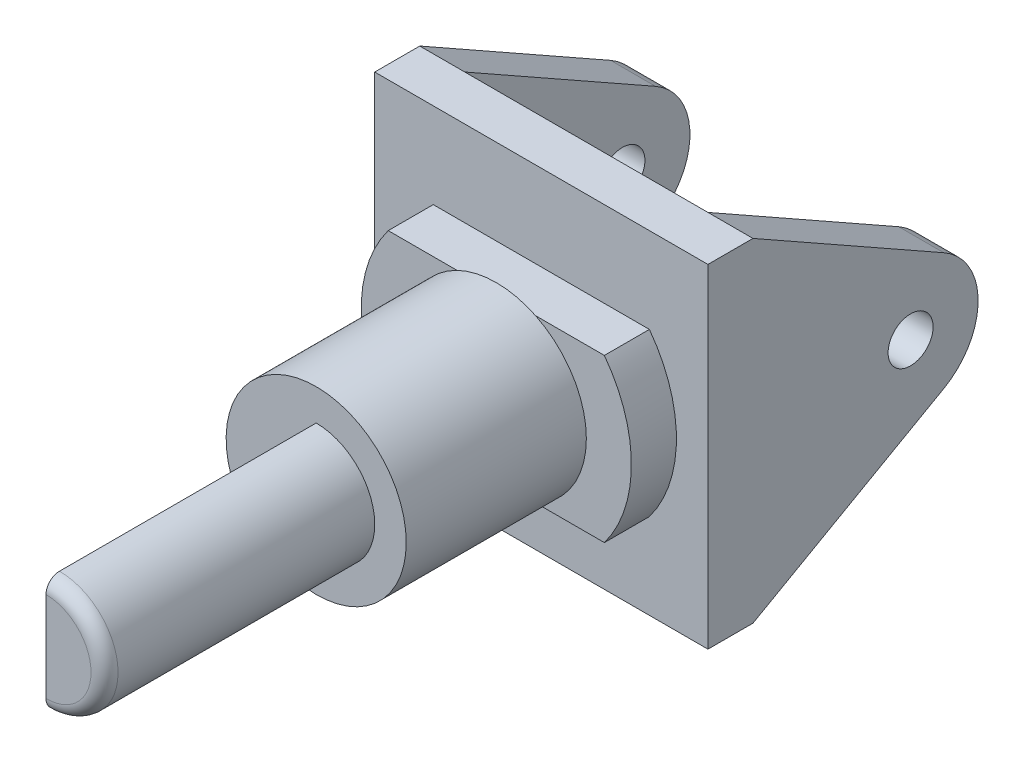
ISO-10303-21;
HEADER;
FILE_DESCRIPTION(('STEP AP214'),'2;1');
FILE_NAME('part.step','',(''),(''),'','','');
FILE_SCHEMA(('AUTOMOTIVE_DESIGN { 1 0 10303 214 1 1 1 1 }'));
ENDSEC;
DATA;
#1=APPLICATION_CONTEXT('core data for automotive mechanical design processes');
#2=APPLICATION_PROTOCOL_DEFINITION('international standard','automotive_design',2000,#1);
#3=PRODUCT_CONTEXT('',#1,'mechanical');
#4=PRODUCT('Part','Part','',(#3));
#5=PRODUCT_RELATED_PRODUCT_CATEGORY('part','',(#4));
#6=PRODUCT_DEFINITION_FORMATION('','',#4);
#7=PRODUCT_DEFINITION_CONTEXT('part definition',#1,'design');
#8=PRODUCT_DEFINITION('design','',#6,#7);
#9=PRODUCT_DEFINITION_SHAPE('','',#8);
#10=(LENGTH_UNIT() NAMED_UNIT(*) SI_UNIT(.MILLI.,.METRE.));
#11=(NAMED_UNIT(*) PLANE_ANGLE_UNIT() SI_UNIT($,.RADIAN.));
#12=(NAMED_UNIT(*) SI_UNIT($,.STERADIAN.) SOLID_ANGLE_UNIT());
#13=UNCERTAINTY_MEASURE_WITH_UNIT(LENGTH_MEASURE(1.E-05),#10,'distance_accuracy_value','');
#14=(GEOMETRIC_REPRESENTATION_CONTEXT(3) GLOBAL_UNCERTAINTY_ASSIGNED_CONTEXT((#13)) GLOBAL_UNIT_ASSIGNED_CONTEXT((#10,
#11,#12)) REPRESENTATION_CONTEXT('',''));
#15=CARTESIAN_POINT('',(0.,0.,0.));
#16=DIRECTION('',(0.,0.,1.));
#17=DIRECTION('',(1.,0.,0.));
#18=AXIS2_PLACEMENT_3D('',#15,#16,#17);
#19=CARTESIAN_POINT('',(0.,0.,-10.));
#20=DIRECTION('',(0.,0.,-1.));
#21=DIRECTION('',(-1.,0.,0.));
#22=AXIS2_PLACEMENT_3D('',#19,#20,#21);
#23=PLANE('',#22);
#24=DIRECTION('',(-1.,0.,0.));
#25=VECTOR('',#24,1.);
#26=CARTESIAN_POINT('',(37.,-37.,-10.));
#27=LINE('',#26,#25);
#28=CARTESIAN_POINT('',(27.,-37.,-10.));
#29=VERTEX_POINT('',#28);
#30=CARTESIAN_POINT('',(-27.,-37.,-10.));
#31=VERTEX_POINT('',#30);
#32=EDGE_CURVE('E238',#29,#31,#27,.T.);
#33=ORIENTED_EDGE('',*,*,#32,.T.);
#34=DIRECTION('',(0.,-1.,0.));
#35=VECTOR('',#34,1.);
#36=CARTESIAN_POINT('',(-27.,37.,-10.));
#37=LINE('',#36,#35);
#38=CARTESIAN_POINT('',(-27.,37.,-10.));
#39=VERTEX_POINT('',#38);
#40=EDGE_CURVE('E54',#39,#31,#37,.T.);
#41=ORIENTED_EDGE('',*,*,#40,.F.);
#42=DIRECTION('',(1.,0.,0.));
#43=VECTOR('',#42,1.);
#44=CARTESIAN_POINT('',(37.,37.,-10.));
#45=LINE('',#44,#43);
#46=CARTESIAN_POINT('',(27.,37.,-10.));
#47=VERTEX_POINT('',#46);
#48=EDGE_CURVE('E237',#39,#47,#45,.T.);
#49=ORIENTED_EDGE('',*,*,#48,.T.);
#50=DIRECTION('',(0.,-1.,0.));
#51=VECTOR('',#50,1.);
#52=CARTESIAN_POINT('',(27.,37.,-10.));
#53=LINE('',#52,#51);
#54=EDGE_CURVE('E208',#47,#29,#53,.T.);
#55=ORIENTED_EDGE('',*,*,#54,.T.);
#56=EDGE_LOOP('',(#33,#41,#49,#55));
#57=FACE_BOUND('',#56,.T.);
#58=ADVANCED_FACE('F39',(#57),#23,.T.);
#59=CARTESIAN_POINT('',(0.,0.,110.));
#60=DIRECTION('',(0.,0.,-1.));
#61=DIRECTION('',(-1.,0.,0.));
#62=AXIS2_PLACEMENT_3D('',#59,#60,#61);
#63=CYLINDRICAL_SURFACE('',#62,13.);
#64=DIRECTION('',(0.,0.,-1.));
#65=VECTOR('',#64,1.);
#66=CARTESIAN_POINT('',(0.,13.,110.));
#67=LINE('',#66,#65);
#68=CARTESIAN_POINT('',(0.,13.,107.));
#69=VERTEX_POINT('',#68);
#70=CARTESIAN_POINT('',(0.,13.,50.));
#71=VERTEX_POINT('',#70);
#72=EDGE_CURVE('E269',#69,#71,#67,.T.);
#73=ORIENTED_EDGE('',*,*,#72,.F.);
#74=CARTESIAN_POINT('',(0.,0.,107.));
#75=DIRECTION('',(0.,0.,1.));
#76=DIRECTION('',(1.,0.,0.));
#77=AXIS2_PLACEMENT_3D('',#74,#75,#76);
#78=CIRCLE('',#77,13.);
#79=CARTESIAN_POINT('',(0.,-13.,107.));
#80=VERTEX_POINT('',#79);
#81=EDGE_CURVE('E325',#69,#80,#78,.F.);
#82=ORIENTED_EDGE('',*,*,#81,.T.);
#83=DIRECTION('',(0.,0.,-1.));
#84=VECTOR('',#83,1.);
#85=CARTESIAN_POINT('',(0.,-13.,110.));
#86=LINE('',#85,#84);
#87=CARTESIAN_POINT('',(0.,-13.,50.));
#88=VERTEX_POINT('',#87);
#89=EDGE_CURVE('E272',#88,#80,#86,.F.);
#90=ORIENTED_EDGE('',*,*,#89,.F.);
#91=CARTESIAN_POINT('',(0.,0.,50.));
#92=DIRECTION('',(0.,0.,1.));
#93=DIRECTION('',(1.,0.,0.));
#94=AXIS2_PLACEMENT_3D('',#91,#92,#93);
#95=CIRCLE('',#94,13.);
#96=EDGE_CURVE('E274',#88,#71,#95,.T.);
#97=ORIENTED_EDGE('',*,*,#96,.T.);
#98=EDGE_LOOP('',(#73,#82,#90,#97));
#99=FACE_BOUND('',#98,.T.);
#100=ADVANCED_FACE('F337',(#99),#63,.T.);
#101=CARTESIAN_POINT('',(0.,0.,110.));
#102=DIRECTION('',(0.,0.,1.));
#103=DIRECTION('',(1.,0.,0.));
#104=AXIS2_PLACEMENT_3D('',#101,#102,#103);
#105=PLANE('',#104);
#106=CARTESIAN_POINT('',(0.,0.,110.));
#107=DIRECTION('',(0.,0.,1.));
#108=DIRECTION('',(1.,0.,0.));
#109=AXIS2_PLACEMENT_3D('',#106,#107,#108);
#110=CIRCLE('',#109,10.);
#111=CARTESIAN_POINT('',(0.,-10.,110.));
#112=VERTEX_POINT('',#111);
#113=CARTESIAN_POINT('',(0.,10.,110.));
#114=VERTEX_POINT('',#113);
#115=EDGE_CURVE('E280',#112,#114,#110,.T.);
#116=ORIENTED_EDGE('',*,*,#115,.T.);
#117=DIRECTION('',(0.,-1.,0.));
#118=VECTOR('',#117,1.);
#119=CARTESIAN_POINT('',(0.,0.,110.));
#120=LINE('',#119,#118);
#121=EDGE_CURVE('E268',#114,#112,#120,.T.);
#122=ORIENTED_EDGE('',*,*,#121,.T.);
#123=EDGE_LOOP('',(#116,#122));
#124=FACE_BOUND('',#123,.T.);
#125=ADVANCED_FACE('F335',(#124),#105,.T.);
#126=CARTESIAN_POINT('',(0.,0.,107.));
#127=DIRECTION('',(0.,0.,1.));
#128=DIRECTION('',(1.,0.,0.));
#129=AXIS2_PLACEMENT_3D('',#126,#127,#128);
#130=TOROIDAL_SURFACE('',#129,10.,3.);
#131=ORIENTED_EDGE('',*,*,#115,.F.);
#132=CARTESIAN_POINT('',(0.,-10.,107.));
#133=DIRECTION('',(-1.,0.,0.));
#134=DIRECTION('',(0.,0.,1.));
#135=AXIS2_PLACEMENT_3D('',#132,#133,#134);
#136=CIRCLE('',#135,3.);
#137=EDGE_CURVE('E11',#112,#80,#136,.F.);
#138=ORIENTED_EDGE('',*,*,#137,.T.);
#139=ORIENTED_EDGE('',*,*,#81,.F.);
#140=CARTESIAN_POINT('',(0.,10.,107.));
#141=DIRECTION('',(-1.,0.,0.));
#142=DIRECTION('',(0.,0.,1.));
#143=AXIS2_PLACEMENT_3D('',#140,#141,#142);
#144=CIRCLE('',#143,3.);
#145=EDGE_CURVE('E48',#69,#114,#144,.F.);
#146=ORIENTED_EDGE('',*,*,#145,.T.);
#147=EDGE_LOOP('',(#131,#138,#139,#146));
#148=FACE_BOUND('',#147,.T.);
#149=ADVANCED_FACE('F41',(#148),#130,.T.);
#150=CARTESIAN_POINT('',(0.,0.,10.));
#151=DIRECTION('',(0.,0.,1.));
#152=DIRECTION('',(1.,0.,0.));
#153=AXIS2_PLACEMENT_3D('',#150,#151,#152);
#154=PLANE('',#153);
#155=CARTESIAN_POINT('',(0.,0.,10.));
#156=DIRECTION('',(0.,0.,1.));
#157=DIRECTION('',(1.,0.,0.));
#158=AXIS2_PLACEMENT_3D('',#155,#156,#157);
#159=CIRCLE('',#158,20.);
#160=CARTESIAN_POINT('',(-8.71779788708135,18.,10.));
#161=VERTEX_POINT('',#160);
#162=CARTESIAN_POINT('',(-8.71779788708135,-18.,10.));
#163=VERTEX_POINT('',#162);
#164=EDGE_CURVE('E279',#161,#163,#159,.T.);
#165=ORIENTED_EDGE('',*,*,#164,.F.);
#166=DIRECTION('',(1.,0.,0.));
#167=VECTOR('',#166,1.);
#168=CARTESIAN_POINT('',(0.,18.,10.));
#169=LINE('',#168,#167);
#170=CARTESIAN_POINT('',(-24.,18.,10.));
#171=VERTEX_POINT('',#170);
#172=EDGE_CURVE('E293',#171,#161,#169,.T.);
#173=ORIENTED_EDGE('',*,*,#172,.F.);
#174=CARTESIAN_POINT('',(0.,0.,10.));
#175=DIRECTION('',(0.,0.,1.));
#176=DIRECTION('',(1.,0.,0.));
#177=AXIS2_PLACEMENT_3D('',#174,#175,#176);
#178=CIRCLE('',#177,30.);
#179=CARTESIAN_POINT('',(-24.,-18.,10.));
#180=VERTEX_POINT('',#179);
#181=EDGE_CURVE('E317',#171,#180,#178,.T.);
#182=ORIENTED_EDGE('',*,*,#181,.T.);
#183=DIRECTION('',(-1.,0.,0.));
#184=VECTOR('',#183,1.);
#185=CARTESIAN_POINT('',(0.,-18.,10.));
#186=LINE('',#185,#184);
#187=EDGE_CURVE('E282',#163,#180,#186,.T.);
#188=ORIENTED_EDGE('',*,*,#187,.F.);
#189=EDGE_LOOP('',(#165,#173,#182,#188));
#190=FACE_BOUND('',#189,.T.);
#191=ADVANCED_FACE('F377',(#190),#154,.T.);
#192=CARTESIAN_POINT('',(0.,0.,10.));
#193=DIRECTION('',(0.,0.,-1.));
#194=DIRECTION('',(-1.,0.,0.));
#195=AXIS2_PLACEMENT_3D('',#192,#193,#194);
#196=CYLINDRICAL_SURFACE('',#195,30.);
#197=ORIENTED_EDGE('',*,*,#181,.F.);
#198=DIRECTION('',(0.,0.,1.));
#199=VECTOR('',#198,1.);
#200=CARTESIAN_POINT('',(-24.,18.,0.));
#201=LINE('',#200,#199);
#202=CARTESIAN_POINT('',(-24.,18.,0.));
#203=VERTEX_POINT('',#202);
#204=EDGE_CURVE('E298',#203,#171,#201,.T.);
#205=ORIENTED_EDGE('',*,*,#204,.F.);
#206=CARTESIAN_POINT('',(0.,0.,0.));
#207=DIRECTION('',(0.,0.,1.));
#208=DIRECTION('',(1.,0.,0.));
#209=AXIS2_PLACEMENT_3D('',#206,#207,#208);
#210=CIRCLE('',#209,30.);
#211=CARTESIAN_POINT('',(-24.,-18.,0.));
#212=VERTEX_POINT('',#211);
#213=EDGE_CURVE('E320',#203,#212,#210,.T.);
#214=ORIENTED_EDGE('',*,*,#213,.T.);
#215=DIRECTION('',(0.,0.,1.));
#216=VECTOR('',#215,1.);
#217=CARTESIAN_POINT('',(-24.,-18.,0.));
#218=LINE('',#217,#216);
#219=EDGE_CURVE('E307',#212,#180,#218,.T.);
#220=ORIENTED_EDGE('',*,*,#219,.T.);
#221=EDGE_LOOP('',(#197,#205,#214,#220));
#222=FACE_BOUND('',#221,.T.);
#223=ADVANCED_FACE('F382',(#222),#196,.T.);
#224=CARTESIAN_POINT('',(24.,-18.,0.));
#225=VERTEX_POINT('',#224);
#226=CARTESIAN_POINT('',(24.,18.,0.));
#227=VERTEX_POINT('',#226);
#228=EDGE_CURVE('E296',#225,#227,#210,.T.);
#229=ORIENTED_EDGE('',*,*,#228,.T.);
#230=DIRECTION('',(0.,0.,1.));
#231=VECTOR('',#230,1.);
#232=CARTESIAN_POINT('',(24.,18.,0.));
#233=LINE('',#232,#231);
#234=CARTESIAN_POINT('',(24.,18.,10.));
#235=VERTEX_POINT('',#234);
#236=EDGE_CURVE('E287',#227,#235,#233,.T.);
#237=ORIENTED_EDGE('',*,*,#236,.T.);
#238=CARTESIAN_POINT('',(24.,-18.,10.));
#239=VERTEX_POINT('',#238);
#240=EDGE_CURVE('E312',#239,#235,#178,.T.);
#241=ORIENTED_EDGE('',*,*,#240,.F.);
#242=DIRECTION('',(0.,0.,1.));
#243=VECTOR('',#242,1.);
#244=CARTESIAN_POINT('',(24.,-18.,0.));
#245=LINE('',#244,#243);
#246=EDGE_CURVE('E302',#225,#239,#245,.T.);
#247=ORIENTED_EDGE('',*,*,#246,.F.);
#248=EDGE_LOOP('',(#229,#237,#241,#247));
#249=FACE_BOUND('',#248,.T.);
#250=ADVANCED_FACE('F361',(#249),#196,.T.);
#251=CARTESIAN_POINT('',(8.71779788708135,-18.,10.));
#252=VERTEX_POINT('',#251);
#253=CARTESIAN_POINT('',(8.71779788708135,18.,10.));
#254=VERTEX_POINT('',#253);
#255=EDGE_CURVE('E288',#252,#254,#159,.T.);
#256=ORIENTED_EDGE('',*,*,#255,.F.);
#257=EDGE_CURVE('E304',#239,#252,#186,.T.);
#258=ORIENTED_EDGE('',*,*,#257,.F.);
#259=ORIENTED_EDGE('',*,*,#240,.T.);
#260=EDGE_CURVE('E294',#254,#235,#169,.T.);
#261=ORIENTED_EDGE('',*,*,#260,.F.);
#262=EDGE_LOOP('',(#256,#258,#259,#261));
#263=FACE_BOUND('',#262,.T.);
#264=ADVANCED_FACE('F370',(#263),#154,.T.);
#265=CARTESIAN_POINT('',(0.,-18.,0.));
#266=DIRECTION('',(0.,1.,0.));
#267=DIRECTION('',(0.,0.,1.));
#268=AXIS2_PLACEMENT_3D('',#265,#266,#267);
#269=PLANE('',#268);
#270=ORIENTED_EDGE('',*,*,#257,.T.);
#271=EDGE_CURVE('E308',#252,#163,#186,.T.);
#272=ORIENTED_EDGE('',*,*,#271,.T.);
#273=ORIENTED_EDGE('',*,*,#187,.T.);
#274=ORIENTED_EDGE('',*,*,#219,.F.);
#275=DIRECTION('',(-1.,0.,0.));
#276=VECTOR('',#275,1.);
#277=CARTESIAN_POINT('',(0.,-18.,0.));
#278=LINE('',#277,#276);
#279=EDGE_CURVE('E301',#225,#212,#278,.T.);
#280=ORIENTED_EDGE('',*,*,#279,.F.);
#281=ORIENTED_EDGE('',*,*,#246,.T.);
#282=EDGE_LOOP('',(#270,#272,#273,#274,#280,#281));
#283=FACE_BOUND('',#282,.T.);
#284=ADVANCED_FACE('F371',(#283),#269,.F.);
#285=CARTESIAN_POINT('',(0.,18.,0.));
#286=DIRECTION('',(0.,-1.,0.));
#287=DIRECTION('',(0.,0.,-1.));
#288=AXIS2_PLACEMENT_3D('',#285,#286,#287);
#289=PLANE('',#288);
#290=ORIENTED_EDGE('',*,*,#172,.T.);
#291=EDGE_CURVE('E295',#161,#254,#169,.T.);
#292=ORIENTED_EDGE('',*,*,#291,.T.);
#293=ORIENTED_EDGE('',*,*,#260,.T.);
#294=ORIENTED_EDGE('',*,*,#236,.F.);
#295=DIRECTION('',(1.,0.,0.));
#296=VECTOR('',#295,1.);
#297=CARTESIAN_POINT('',(0.,18.,0.));
#298=LINE('',#297,#296);
#299=EDGE_CURVE('E290',#203,#227,#298,.T.);
#300=ORIENTED_EDGE('',*,*,#299,.F.);
#301=ORIENTED_EDGE('',*,*,#204,.T.);
#302=EDGE_LOOP('',(#290,#292,#293,#294,#300,#301));
#303=FACE_BOUND('',#302,.T.);
#304=ADVANCED_FACE('F360',(#303),#289,.F.);
#305=CARTESIAN_POINT('',(0.,0.,10.));
#306=DIRECTION('',(0.,0.,1.));
#307=DIRECTION('',(1.,0.,0.));
#308=AXIS2_PLACEMENT_3D('',#305,#306,#307);
#309=PLANE('',#308);
#310=ORIENTED_EDGE('',*,*,#291,.F.);
#311=EDGE_CURVE('E284',#254,#161,#159,.T.);
#312=ORIENTED_EDGE('',*,*,#311,.F.);
#313=EDGE_LOOP('',(#310,#312));
#314=FACE_BOUND('',#313,.T.);
#315=ADVANCED_FACE('F348',(#314),#309,.F.);
#316=CARTESIAN_POINT('',(0.,0.,50.));
#317=DIRECTION('',(0.,0.,-1.));
#318=DIRECTION('',(-1.,0.,0.));
#319=AXIS2_PLACEMENT_3D('',#316,#317,#318);
#320=CYLINDRICAL_SURFACE('',#319,20.);
#321=CARTESIAN_POINT('',(0.,0.,50.));
#322=DIRECTION('',(0.,0.,1.));
#323=DIRECTION('',(1.,0.,0.));
#324=AXIS2_PLACEMENT_3D('',#321,#322,#323);
#325=CIRCLE('',#324,20.);
#326=CARTESIAN_POINT('',(20.,0.,50.));
#327=VERTEX_POINT('',#326);
#328=EDGE_CURVE('E276',#327,#327,#325,.T.);
#329=ORIENTED_EDGE('',*,*,#328,.F.);
#330=EDGE_LOOP('',(#329));
#331=FACE_BOUND('',#330,.T.);
#332=ORIENTED_EDGE('',*,*,#311,.T.);
#333=ORIENTED_EDGE('',*,*,#164,.T.);
#334=EDGE_CURVE('E271',#163,#252,#159,.T.);
#335=ORIENTED_EDGE('',*,*,#334,.T.);
#336=ORIENTED_EDGE('',*,*,#255,.T.);
#337=EDGE_LOOP('',(#332,#333,#335,#336));
#338=FACE_BOUND('',#337,.T.);
#339=ADVANCED_FACE('F344',(#331,#338),#320,.T.);
#340=CARTESIAN_POINT('',(0.,0.,50.));
#341=DIRECTION('',(0.,0.,1.));
#342=DIRECTION('',(1.,0.,0.));
#343=AXIS2_PLACEMENT_3D('',#340,#341,#342);
#344=PLANE('',#343);
#345=DIRECTION('',(0.,1.,0.));
#346=VECTOR('',#345,1.);
#347=CARTESIAN_POINT('',(0.,20.0222914024367,50.));
#348=LINE('',#347,#346);
#349=EDGE_CURVE('E264',#88,#71,#348,.T.);
#350=ORIENTED_EDGE('',*,*,#349,.T.);
#351=ORIENTED_EDGE('',*,*,#96,.F.);
#352=EDGE_LOOP('',(#350,#351));
#353=FACE_BOUND('',#352,.T.);
#354=ORIENTED_EDGE('',*,*,#328,.T.);
#355=EDGE_LOOP('',(#354));
#356=FACE_BOUND('',#355,.T.);
#357=ADVANCED_FACE('F339',(#353,#356),#344,.T.);
#358=ORIENTED_EDGE('',*,*,#271,.F.);
#359=ORIENTED_EDGE('',*,*,#334,.F.);
#360=EDGE_LOOP('',(#358,#359));
#361=FACE_BOUND('',#360,.T.);
#362=ADVANCED_FACE('F345',(#361),#309,.F.);
#363=CARTESIAN_POINT('',(0.,0.,0.));
#364=DIRECTION('',(-1.,0.,0.));
#365=DIRECTION('',(0.,0.,1.));
#366=AXIS2_PLACEMENT_3D('',#363,#364,#365);
#367=PLANE('',#366);
#368=ORIENTED_EDGE('',*,*,#89,.T.);
#369=ORIENTED_EDGE('',*,*,#137,.F.);
#370=ORIENTED_EDGE('',*,*,#121,.F.);
#371=ORIENTED_EDGE('',*,*,#145,.F.);
#372=ORIENTED_EDGE('',*,*,#72,.T.);
#373=ORIENTED_EDGE('',*,*,#349,.F.);
#374=EDGE_LOOP('',(#368,#369,#370,#371,#372,#373));
#375=FACE_BOUND('',#374,.T.);
#376=ADVANCED_FACE('F331',(#375),#367,.T.);
#377=CARTESIAN_POINT('',(-37.,37.,-10.));
#378=DIRECTION('',(1.,0.,0.));
#379=DIRECTION('',(0.,1.,0.));
#380=AXIS2_PLACEMENT_3D('',#377,#378,#379);
#381=PLANE('',#380);
#382=CARTESIAN_POINT('',(-37.,0.,-45.));
#383=DIRECTION('',(1.,0.,0.));
#384=DIRECTION('',(0.,0.,-1.));
#385=AXIS2_PLACEMENT_3D('',#382,#383,#384);
#386=CIRCLE('',#385,5.);
#387=CARTESIAN_POINT('',(-37.,0.,-50.));
#388=VERTEX_POINT('',#387);
#389=EDGE_CURVE('E615',#388,#388,#386,.T.);
#390=ORIENTED_EDGE('',*,*,#389,.T.);
#391=EDGE_LOOP('',(#390));
#392=FACE_BOUND('',#391,.T.);
#393=DIRECTION('',(0.,1.,0.));
#394=VECTOR('',#393,1.);
#395=CARTESIAN_POINT('',(-37.,37.,0.));
#396=LINE('',#395,#394);
#397=CARTESIAN_POINT('',(-37.,-37.,0.));
#398=VERTEX_POINT('',#397);
#399=CARTESIAN_POINT('',(-37.,37.,0.));
#400=VERTEX_POINT('',#399);
#401=EDGE_CURVE('E231',#398,#400,#396,.T.);
#402=ORIENTED_EDGE('',*,*,#401,.T.);
#403=DIRECTION('',(0.,0.,1.));
#404=VECTOR('',#403,1.);
#405=CARTESIAN_POINT('',(-37.,37.,-10.));
#406=LINE('',#405,#404);
#407=CARTESIAN_POINT('',(-37.,37.,-10.));
#408=VERTEX_POINT('',#407);
#409=EDGE_CURVE('E258',#408,#400,#406,.T.);
#410=ORIENTED_EDGE('',*,*,#409,.F.);
#411=DIRECTION('',(0.,0.491857302042567,0.870675826256482));
#412=VECTOR('',#411,1.);
#413=CARTESIAN_POINT('',(-37.,37.,-10.));
#414=LINE('',#413,#412);
#415=CARTESIAN_POINT('',(-37.,13.0601373938472,-52.3778595306385));
#416=VERTEX_POINT('',#415);
#417=EDGE_CURVE('E205',#416,#408,#414,.T.);
#418=ORIENTED_EDGE('',*,*,#417,.F.);
#419=CARTESIAN_POINT('',(-37.,0.,-45.));
#420=DIRECTION('',(1.,0.,0.));
#421=DIRECTION('',(0.,0.,-1.));
#422=AXIS2_PLACEMENT_3D('',#419,#420,#421);
#423=CIRCLE('',#422,15.);
#424=CARTESIAN_POINT('',(-37.,-13.0601373938472,-52.3778595306385));
#425=VERTEX_POINT('',#424);
#426=EDGE_CURVE('E189',#425,#416,#423,.T.);
#427=ORIENTED_EDGE('',*,*,#426,.F.);
#428=DIRECTION('',(0.,0.491857302042566,-0.870675826256482));
#429=VECTOR('',#428,1.);
#430=CARTESIAN_POINT('',(-37.,-37.,-10.));
#431=LINE('',#430,#429);
#432=CARTESIAN_POINT('',(-37.,-37.,-10.));
#433=VERTEX_POINT('',#432);
#434=EDGE_CURVE('E197',#433,#425,#431,.T.);
#435=ORIENTED_EDGE('',*,*,#434,.F.);
#436=DIRECTION('',(0.,0.,1.));
#437=VECTOR('',#436,1.);
#438=CARTESIAN_POINT('',(-37.,-37.,-10.));
#439=LINE('',#438,#437);
#440=EDGE_CURVE('E243',#433,#398,#439,.T.);
#441=ORIENTED_EDGE('',*,*,#440,.T.);
#442=EDGE_LOOP('',(#402,#410,#418,#427,#435,#441));
#443=FACE_BOUND('',#442,.T.);
#444=ADVANCED_FACE('F398',(#392,#443),#381,.F.);
#445=CARTESIAN_POINT('',(37.,37.,-10.));
#446=DIRECTION('',(0.,-1.,0.));
#447=DIRECTION('',(1.,0.,0.));
#448=AXIS2_PLACEMENT_3D('',#445,#446,#447);
#449=PLANE('',#448);
#450=DIRECTION('',(1.,0.,0.));
#451=VECTOR('',#450,1.);
#452=CARTESIAN_POINT('',(37.,37.,0.));
#453=LINE('',#452,#451);
#454=CARTESIAN_POINT('',(37.,37.,0.));
#455=VERTEX_POINT('',#454);
#456=EDGE_CURVE('E246',#400,#455,#453,.T.);
#457=ORIENTED_EDGE('',*,*,#456,.T.);
#458=DIRECTION('',(0.,0.,1.));
#459=VECTOR('',#458,1.);
#460=CARTESIAN_POINT('',(37.,37.,-10.));
#461=LINE('',#460,#459);
#462=CARTESIAN_POINT('',(37.,37.,-10.));
#463=VERTEX_POINT('',#462);
#464=EDGE_CURVE('E260',#463,#455,#461,.T.);
#465=ORIENTED_EDGE('',*,*,#464,.F.);
#466=DIRECTION('',(1.,0.,0.));
#467=VECTOR('',#466,1.);
#468=CARTESIAN_POINT('',(27.,37.,-10.));
#469=LINE('',#468,#467);
#470=EDGE_CURVE('E233',#47,#463,#469,.T.);
#471=ORIENTED_EDGE('',*,*,#470,.F.);
#472=ORIENTED_EDGE('',*,*,#48,.F.);
#473=EDGE_CURVE('E193',#408,#39,#45,.T.);
#474=ORIENTED_EDGE('',*,*,#473,.F.);
#475=ORIENTED_EDGE('',*,*,#409,.T.);
#476=EDGE_LOOP('',(#457,#465,#471,#472,#474,#475));
#477=FACE_BOUND('',#476,.T.);
#478=ADVANCED_FACE('F407',(#477),#449,.F.);
#479=CARTESIAN_POINT('',(37.,37.,-10.));
#480=DIRECTION('',(-1.,0.,0.));
#481=DIRECTION('',(0.,0.,1.));
#482=AXIS2_PLACEMENT_3D('',#479,#480,#481);
#483=PLANE('',#482);
#484=CARTESIAN_POINT('',(37.,0.,-45.));
#485=DIRECTION('',(1.,0.,0.));
#486=DIRECTION('',(0.,0.,-1.));
#487=AXIS2_PLACEMENT_3D('',#484,#485,#486);
#488=CIRCLE('',#487,5.);
#489=CARTESIAN_POINT('',(37.,0.,-50.));
#490=VERTEX_POINT('',#489);
#491=EDGE_CURVE('E609',#490,#490,#488,.T.);
#492=ORIENTED_EDGE('',*,*,#491,.F.);
#493=EDGE_LOOP('',(#492));
#494=FACE_BOUND('',#493,.T.);
#495=DIRECTION('',(0.,-1.,0.));
#496=VECTOR('',#495,1.);
#497=CARTESIAN_POINT('',(37.,37.,0.));
#498=LINE('',#497,#496);
#499=CARTESIAN_POINT('',(37.,-37.,0.));
#500=VERTEX_POINT('',#499);
#501=EDGE_CURVE('E247',#455,#500,#498,.T.);
#502=ORIENTED_EDGE('',*,*,#501,.T.);
#503=DIRECTION('',(0.,0.,1.));
#504=VECTOR('',#503,1.);
#505=CARTESIAN_POINT('',(37.,-37.,-10.));
#506=LINE('',#505,#504);
#507=CARTESIAN_POINT('',(37.,-37.,-10.));
#508=VERTEX_POINT('',#507);
#509=EDGE_CURVE('E251',#508,#500,#506,.T.);
#510=ORIENTED_EDGE('',*,*,#509,.F.);
#511=DIRECTION('',(0.,0.491857302042566,-0.870675826256482));
#512=VECTOR('',#511,1.);
#513=CARTESIAN_POINT('',(37.,-37.,-10.));
#514=LINE('',#513,#512);
#515=CARTESIAN_POINT('',(37.,-13.0601373938472,-52.3778595306385));
#516=VERTEX_POINT('',#515);
#517=EDGE_CURVE('E206',#508,#516,#514,.T.);
#518=ORIENTED_EDGE('',*,*,#517,.T.);
#519=CARTESIAN_POINT('',(37.,0.,-45.));
#520=DIRECTION('',(1.,0.,0.));
#521=DIRECTION('',(0.,0.,-1.));
#522=AXIS2_PLACEMENT_3D('',#519,#520,#521);
#523=CIRCLE('',#522,15.);
#524=CARTESIAN_POINT('',(37.,13.0601373938472,-52.3778595306385));
#525=VERTEX_POINT('',#524);
#526=EDGE_CURVE('E228',#516,#525,#523,.T.);
#527=ORIENTED_EDGE('',*,*,#526,.T.);
#528=DIRECTION('',(0.,0.491857302042567,0.870675826256482));
#529=VECTOR('',#528,1.);
#530=CARTESIAN_POINT('',(37.,37.,-10.));
#531=LINE('',#530,#529);
#532=EDGE_CURVE('E211',#525,#463,#531,.T.);
#533=ORIENTED_EDGE('',*,*,#532,.T.);
#534=ORIENTED_EDGE('',*,*,#464,.T.);
#535=EDGE_LOOP('',(#502,#510,#518,#527,#533,#534));
#536=FACE_BOUND('',#535,.T.);
#537=ADVANCED_FACE('F402',(#494,#536),#483,.F.);
#538=CARTESIAN_POINT('',(37.,-37.,-10.));
#539=DIRECTION('',(0.,1.,0.));
#540=DIRECTION('',(0.,0.,1.));
#541=AXIS2_PLACEMENT_3D('',#538,#539,#540);
#542=PLANE('',#541);
#543=DIRECTION('',(-1.,0.,0.));
#544=VECTOR('',#543,1.);
#545=CARTESIAN_POINT('',(37.,-37.,0.));
#546=LINE('',#545,#544);
#547=EDGE_CURVE('E249',#500,#398,#546,.T.);
#548=ORIENTED_EDGE('',*,*,#547,.T.);
#549=ORIENTED_EDGE('',*,*,#440,.F.);
#550=DIRECTION('',(-1.,0.,0.));
#551=VECTOR('',#550,1.);
#552=CARTESIAN_POINT('',(-27.,-37.,-10.));
#553=LINE('',#552,#551);
#554=EDGE_CURVE('E64',#31,#433,#553,.T.);
#555=ORIENTED_EDGE('',*,*,#554,.F.);
#556=ORIENTED_EDGE('',*,*,#32,.F.);
#557=EDGE_CURVE('E239',#508,#29,#27,.T.);
#558=ORIENTED_EDGE('',*,*,#557,.F.);
#559=ORIENTED_EDGE('',*,*,#509,.T.);
#560=EDGE_LOOP('',(#548,#549,#555,#556,#558,#559));
#561=FACE_BOUND('',#560,.T.);
#562=ADVANCED_FACE('F386',(#561),#542,.F.);
#563=CARTESIAN_POINT('',(0.,0.,0.));
#564=DIRECTION('',(0.,0.,-1.));
#565=DIRECTION('',(-1.,0.,0.));
#566=AXIS2_PLACEMENT_3D('',#563,#564,#565);
#567=PLANE('',#566);
#568=ORIENTED_EDGE('',*,*,#213,.F.);
#569=ORIENTED_EDGE('',*,*,#299,.T.);
#570=ORIENTED_EDGE('',*,*,#228,.F.);
#571=ORIENTED_EDGE('',*,*,#279,.T.);
#572=EDGE_LOOP('',(#568,#569,#570,#571));
#573=FACE_BOUND('',#572,.T.);
#574=ORIENTED_EDGE('',*,*,#401,.F.);
#575=ORIENTED_EDGE('',*,*,#547,.F.);
#576=ORIENTED_EDGE('',*,*,#501,.F.);
#577=ORIENTED_EDGE('',*,*,#456,.F.);
#578=EDGE_LOOP('',(#574,#575,#576,#577));
#579=FACE_BOUND('',#578,.T.);
#580=ADVANCED_FACE('F383',(#573,#579),#567,.F.);
#581=CARTESIAN_POINT('',(27.,37.,-10.));
#582=DIRECTION('',(0.,0.870675826256482,-0.491857302042566));
#583=DIRECTION('',(0.,0.491857302042566,0.870675826256482));
#584=AXIS2_PLACEMENT_3D('',#581,#582,#583);
#585=PLANE('',#584);
#586=ORIENTED_EDGE('',*,*,#532,.F.);
#587=DIRECTION('',(1.,0.,0.));
#588=VECTOR('',#587,1.);
#589=CARTESIAN_POINT('',(27.,13.0601373938472,-52.3778595306385));
#590=LINE('',#589,#588);
#591=CARTESIAN_POINT('',(27.,13.0601373938472,-52.3778595306385));
#592=VERTEX_POINT('',#591);
#593=EDGE_CURVE('E234',#592,#525,#590,.T.);
#594=ORIENTED_EDGE('',*,*,#593,.F.);
#595=DIRECTION('',(0.,0.491857302042567,0.870675826256482));
#596=VECTOR('',#595,1.);
#597=CARTESIAN_POINT('',(27.,37.,-10.));
#598=LINE('',#597,#596);
#599=EDGE_CURVE('E220',#592,#47,#598,.T.);
#600=ORIENTED_EDGE('',*,*,#599,.T.);
#601=ORIENTED_EDGE('',*,*,#470,.T.);
#602=EDGE_LOOP('',(#586,#594,#600,#601));
#603=FACE_BOUND('',#602,.T.);
#604=ADVANCED_FACE('F389',(#603),#585,.T.);
#605=CARTESIAN_POINT('',(27.,0.,-45.));
#606=DIRECTION('',(1.,0.,0.));
#607=DIRECTION('',(0.,0.,-1.));
#608=AXIS2_PLACEMENT_3D('',#605,#606,#607);
#609=CYLINDRICAL_SURFACE('',#608,15.);
#610=ORIENTED_EDGE('',*,*,#526,.F.);
#611=DIRECTION('',(1.,0.,0.));
#612=VECTOR('',#611,1.);
#613=CARTESIAN_POINT('',(27.,-13.0601373938472,-52.3778595306385));
#614=LINE('',#613,#612);
#615=CARTESIAN_POINT('',(27.,-13.0601373938472,-52.3778595306385));
#616=VERTEX_POINT('',#615);
#617=EDGE_CURVE('E221',#616,#516,#614,.T.);
#618=ORIENTED_EDGE('',*,*,#617,.F.);
#619=CARTESIAN_POINT('',(27.,0.,-45.));
#620=DIRECTION('',(1.,0.,0.));
#621=DIRECTION('',(0.,0.,-1.));
#622=AXIS2_PLACEMENT_3D('',#619,#620,#621);
#623=CIRCLE('',#622,15.);
#624=EDGE_CURVE('E217',#616,#592,#623,.T.);
#625=ORIENTED_EDGE('',*,*,#624,.T.);
#626=ORIENTED_EDGE('',*,*,#593,.T.);
#627=EDGE_LOOP('',(#610,#618,#625,#626));
#628=FACE_BOUND('',#627,.T.);
#629=ADVANCED_FACE('F415',(#628),#609,.T.);
#630=CARTESIAN_POINT('',(27.,-37.,-10.));
#631=DIRECTION('',(0.,-0.870675826256482,-0.491857302042566));
#632=DIRECTION('',(0.,0.491857302042566,-0.870675826256482));
#633=AXIS2_PLACEMENT_3D('',#630,#631,#632);
#634=PLANE('',#633);
#635=ORIENTED_EDGE('',*,*,#517,.F.);
#636=ORIENTED_EDGE('',*,*,#557,.T.);
#637=DIRECTION('',(0.,0.491857302042566,-0.870675826256482));
#638=VECTOR('',#637,1.);
#639=CARTESIAN_POINT('',(27.,-37.,-10.));
#640=LINE('',#639,#638);
#641=EDGE_CURVE('E214',#29,#616,#640,.T.);
#642=ORIENTED_EDGE('',*,*,#641,.T.);
#643=ORIENTED_EDGE('',*,*,#617,.T.);
#644=EDGE_LOOP('',(#635,#636,#642,#643));
#645=FACE_BOUND('',#644,.T.);
#646=ADVANCED_FACE('F420',(#645),#634,.T.);
#647=CARTESIAN_POINT('',(27.,0.,-45.));
#648=DIRECTION('',(1.,0.,0.));
#649=DIRECTION('',(0.,0.,-1.));
#650=AXIS2_PLACEMENT_3D('',#647,#648,#649);
#651=PLANE('',#650);
#652=CARTESIAN_POINT('',(27.,0.,-45.));
#653=DIRECTION('',(1.,0.,0.));
#654=DIRECTION('',(0.,0.,-1.));
#655=AXIS2_PLACEMENT_3D('',#652,#653,#654);
#656=CIRCLE('',#655,5.);
#657=CARTESIAN_POINT('',(27.,0.,-50.));
#658=VERTEX_POINT('',#657);
#659=EDGE_CURVE('E204',#658,#658,#656,.T.);
#660=ORIENTED_EDGE('',*,*,#659,.T.);
#661=EDGE_LOOP('',(#660));
#662=FACE_BOUND('',#661,.T.);
#663=ORIENTED_EDGE('',*,*,#54,.F.);
#664=ORIENTED_EDGE('',*,*,#599,.F.);
#665=ORIENTED_EDGE('',*,*,#624,.F.);
#666=ORIENTED_EDGE('',*,*,#641,.F.);
#667=EDGE_LOOP('',(#663,#664,#665,#666));
#668=FACE_BOUND('',#667,.T.);
#669=ADVANCED_FACE('F408',(#662,#668),#651,.F.);
#670=CARTESIAN_POINT('',(-27.,-37.,-10.));
#671=DIRECTION('',(0.,0.870675826256482,0.491857302042566));
#672=DIRECTION('',(0.,-0.491857302042566,0.870675826256482));
#673=AXIS2_PLACEMENT_3D('',#670,#671,#672);
#674=PLANE('',#673);
#675=ORIENTED_EDGE('',*,*,#434,.T.);
#676=DIRECTION('',(-1.,0.,0.));
#677=VECTOR('',#676,1.);
#678=CARTESIAN_POINT('',(-27.,-13.0601373938472,-52.3778595306385));
#679=LINE('',#678,#677);
#680=CARTESIAN_POINT('',(-27.,-13.0601373938472,-52.3778595306385));
#681=VERTEX_POINT('',#680);
#682=EDGE_CURVE('E195',#681,#425,#679,.T.);
#683=ORIENTED_EDGE('',*,*,#682,.F.);
#684=DIRECTION('',(0.,0.491857302042566,-0.870675826256482));
#685=VECTOR('',#684,1.);
#686=CARTESIAN_POINT('',(-27.,-37.,-10.));
#687=LINE('',#686,#685);
#688=EDGE_CURVE('E177',#31,#681,#687,.T.);
#689=ORIENTED_EDGE('',*,*,#688,.F.);
#690=ORIENTED_EDGE('',*,*,#554,.T.);
#691=EDGE_LOOP('',(#675,#683,#689,#690));
#692=FACE_BOUND('',#691,.T.);
#693=ADVANCED_FACE('F424',(#692),#674,.F.);
#694=CARTESIAN_POINT('',(-27.,0.,-45.));
#695=DIRECTION('',(-1.,0.,0.));
#696=DIRECTION('',(0.,0.,1.));
#697=AXIS2_PLACEMENT_3D('',#694,#695,#696);
#698=CYLINDRICAL_SURFACE('',#697,15.);
#699=ORIENTED_EDGE('',*,*,#426,.T.);
#700=DIRECTION('',(-1.,0.,0.));
#701=VECTOR('',#700,1.);
#702=CARTESIAN_POINT('',(-27.,13.0601373938472,-52.3778595306385));
#703=LINE('',#702,#701);
#704=CARTESIAN_POINT('',(-27.,13.0601373938472,-52.3778595306385));
#705=VERTEX_POINT('',#704);
#706=EDGE_CURVE('E184',#705,#416,#703,.T.);
#707=ORIENTED_EDGE('',*,*,#706,.F.);
#708=CARTESIAN_POINT('',(-27.,0.,-45.));
#709=DIRECTION('',(1.,0.,0.));
#710=DIRECTION('',(0.,0.,-1.));
#711=AXIS2_PLACEMENT_3D('',#708,#709,#710);
#712=CIRCLE('',#711,15.);
#713=EDGE_CURVE('E175',#681,#705,#712,.T.);
#714=ORIENTED_EDGE('',*,*,#713,.F.);
#715=ORIENTED_EDGE('',*,*,#682,.T.);
#716=EDGE_LOOP('',(#699,#707,#714,#715));
#717=FACE_BOUND('',#716,.T.);
#718=ADVANCED_FACE('F187',(#717),#698,.T.);
#719=CARTESIAN_POINT('',(-27.,37.,-10.));
#720=DIRECTION('',(0.,-0.870675826256482,0.491857302042566));
#721=DIRECTION('',(0.,-0.491857302042566,-0.870675826256482));
#722=AXIS2_PLACEMENT_3D('',#719,#720,#721);
#723=PLANE('',#722);
#724=ORIENTED_EDGE('',*,*,#417,.T.);
#725=ORIENTED_EDGE('',*,*,#473,.T.);
#726=DIRECTION('',(0.,0.491857302042567,0.870675826256482));
#727=VECTOR('',#726,1.);
#728=CARTESIAN_POINT('',(-27.,37.,-10.));
#729=LINE('',#728,#727);
#730=EDGE_CURVE('E176',#705,#39,#729,.T.);
#731=ORIENTED_EDGE('',*,*,#730,.F.);
#732=ORIENTED_EDGE('',*,*,#706,.T.);
#733=EDGE_LOOP('',(#724,#725,#731,#732));
#734=FACE_BOUND('',#733,.T.);
#735=ADVANCED_FACE('F191',(#734),#723,.F.);
#736=CARTESIAN_POINT('',(-27.,0.,-45.));
#737=DIRECTION('',(-1.,0.,0.));
#738=DIRECTION('',(0.,0.,-1.));
#739=AXIS2_PLACEMENT_3D('',#736,#737,#738);
#740=PLANE('',#739);
#741=CARTESIAN_POINT('',(-27.,0.,-45.));
#742=DIRECTION('',(-1.,0.,0.));
#743=DIRECTION('',(0.,0.,1.));
#744=AXIS2_PLACEMENT_3D('',#741,#742,#743);
#745=CIRCLE('',#744,5.);
#746=CARTESIAN_POINT('',(-27.,0.,-40.));
#747=VERTEX_POINT('',#746);
#748=EDGE_CURVE('E43',#747,#747,#745,.T.);
#749=ORIENTED_EDGE('',*,*,#748,.T.);
#750=EDGE_LOOP('',(#749));
#751=FACE_BOUND('',#750,.T.);
#752=ORIENTED_EDGE('',*,*,#40,.T.);
#753=ORIENTED_EDGE('',*,*,#688,.T.);
#754=ORIENTED_EDGE('',*,*,#713,.T.);
#755=ORIENTED_EDGE('',*,*,#730,.T.);
#756=EDGE_LOOP('',(#752,#753,#754,#755));
#757=FACE_BOUND('',#756,.T.);
#758=ADVANCED_FACE('F172',(#751,#757),#740,.F.);
#759=CARTESIAN_POINT('',(-37.,0.,-45.));
#760=DIRECTION('',(1.,0.,0.));
#761=DIRECTION('',(0.,0.,-1.));
#762=AXIS2_PLACEMENT_3D('',#759,#760,#761);
#763=CYLINDRICAL_SURFACE('',#762,5.);
#764=ORIENTED_EDGE('',*,*,#389,.F.);
#765=EDGE_LOOP('',(#764));
#766=FACE_BOUND('',#765,.T.);
#767=ORIENTED_EDGE('',*,*,#748,.F.);
#768=EDGE_LOOP('',(#767));
#769=FACE_BOUND('',#768,.T.);
#770=ADVANCED_FACE('F585',(#766,#769),#763,.F.);
#771=ORIENTED_EDGE('',*,*,#491,.T.);
#772=EDGE_LOOP('',(#771));
#773=FACE_BOUND('',#772,.T.);
#774=ORIENTED_EDGE('',*,*,#659,.F.);
#775=EDGE_LOOP('',(#774));
#776=FACE_BOUND('',#775,.T.);
#777=ADVANCED_FACE('F593',(#773,#776),#763,.F.);
#778=CLOSED_SHELL('',(#58,#100,#125,#149,#191,#223,#250,#264,#284,#304,#315,#339,#357,#362,#376,
#444,#478,#537,#562,#580,#604,#629,#646,#669,#693,#718,#735,#758,#770,#777));
#779=MANIFOLD_SOLID_BREP('B2',#778);
#780=ADVANCED_BREP_SHAPE_REPRESENTATION('',(#18,#779),#14);
#781=SHAPE_DEFINITION_REPRESENTATION(#9,#780);
ENDSEC;
END-ISO-10303-21;
